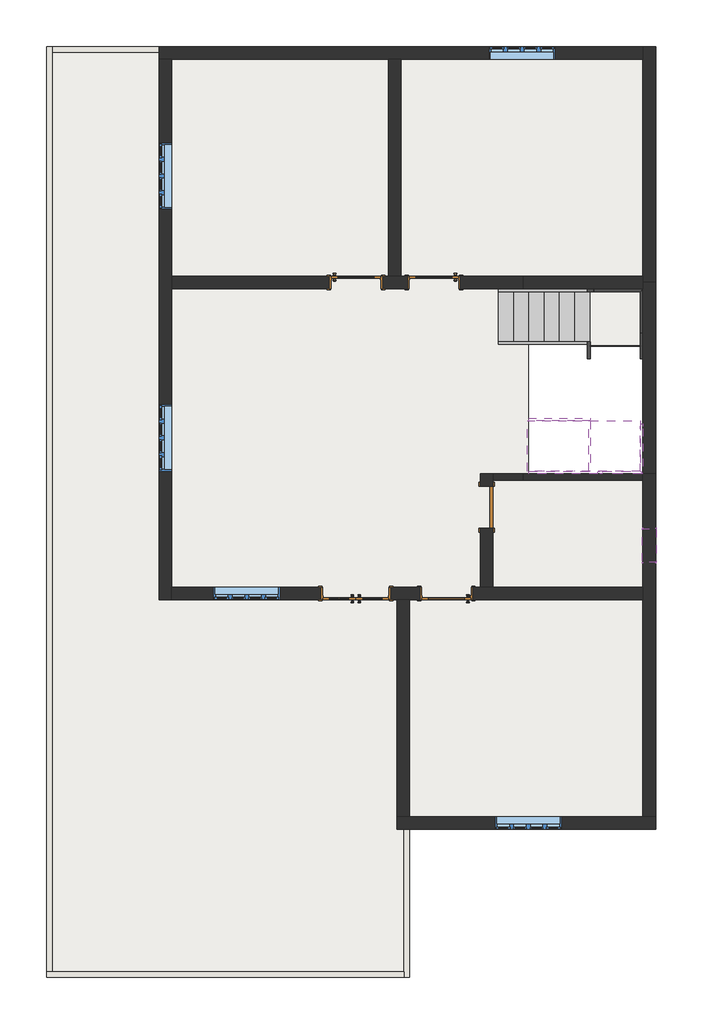
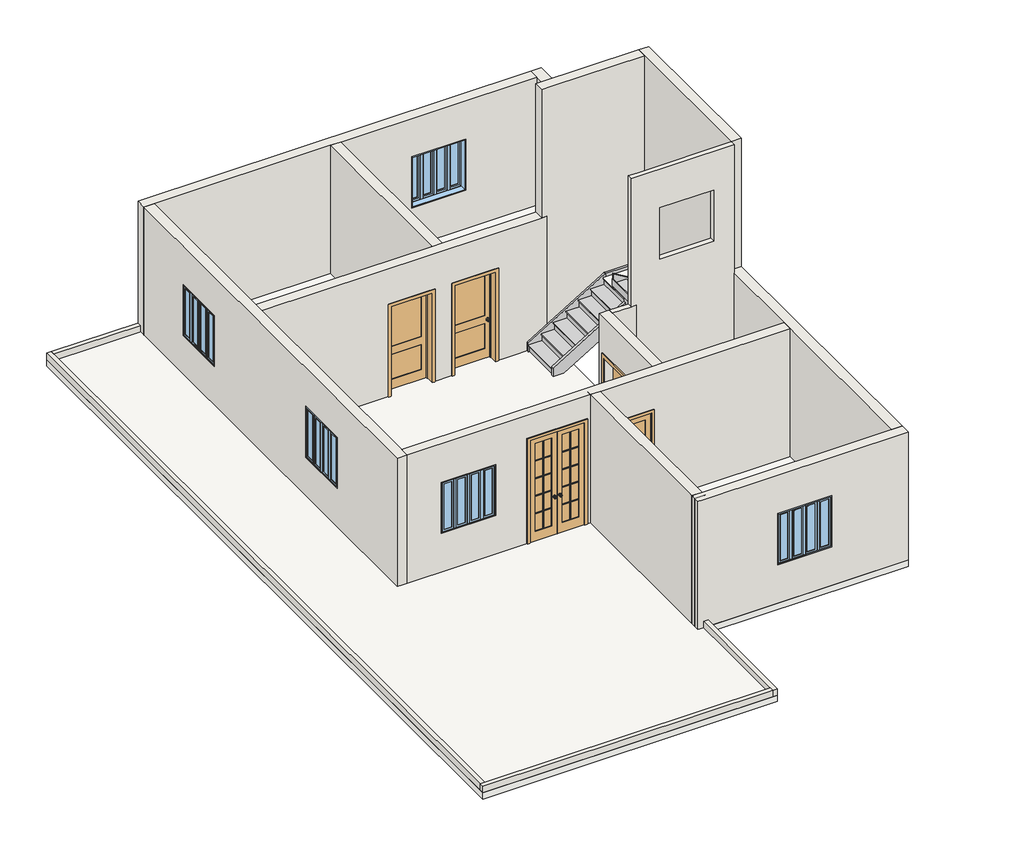
# One storey, incomplete: 18 walls, 10 members, 6 windows, 5 doors, 3 slabs, 3 stair flights, 2 columns.
"""IFC4 building model written with IfcOpenShell, lengths in millimetres."""

from ifc_helpers import new_model, si_unit, frame, origin, place, context, project, spatial, polyline, outline, extrude, faceted_brep, transform, mapped, element, save
from components import door_interior_double_full_glass_wood_4_x_8_door_7870f6d1, door_interior_single_2_panel_wood_3_x_7_door_08fe406f, door_interior_single_2_panel_wood_3_x_7_door_700963f9, door_e31f6e4d, non_monolithic_landing_e7e36702, non_monolithic_landing_8c0399ef, stair_flight_6437b1f2, stair_flight_4bd381d9, stair_flight_f110103f, window_casement_multi_sash_horizontal_4_x_4_8de01852, window_6da96920

model = new_model("IFC4")

# Units and contexts
model_context = context("Model", 3, world=origin())
ifc_project = project(units=[si_unit("LENGTHUNIT", "METRE", prefix="MILLI")], contexts=[model_context])

# Site, building, storey
site = spatial("IfcSite", under=ifc_project)
building = spatial("IfcBuilding", under=site)
storey = spatial("IfcBuildingStorey", under=building, Elevation=3048.0)

# Columns
placement = place(None, origin())
element("IfcColumn", 1, ObjectType="Rectangular Column : 9\" X 9\" COLUMN", at=placement, inside=storey, context=model_context, shape_type="SweptSolid", body=[
    extrude(outline(polyline([(-4334.4608498, -5108.7884134), (-4105.8608498, -5108.7884134), (-4105.8608498, -5222.3884134), (-4334.4608498, -5222.3884134), (-4334.4608498, -5108.7884134)])), frame((0.0, 0.0, 3048.0), z_axis=(0.0, 0.0, 1.0), x_axis=(1.0, 0.0, 0.0)), (0.0, 0.0, 1.0), 3048.0),
])
element("IfcColumn", 2, ObjectType="Rectangular Column : 9\" X 9\" COLUMN", at=placement, inside=storey, context=model_context, shape_type="SweptSolid", body=[
    extrude(outline(polyline([(-4105.8608498, -916.3884134), (-4105.8608498, -1144.9884134), (-4334.4608498, -1144.9884134), (-4334.4608498, -916.3884134), (-4105.8608498, -916.3884134)])), frame((0.0, 0.0, 3048.0), z_axis=(0.0, 0.0, 1.0), x_axis=(1.0, 0.0, 0.0)), (0.0, 0.0, 1.0), 3048.0),
])

# Doors
door_interior_double_full_glass_wood_4_x_8_door_shape = door_interior_double_full_glass_wood_4_x_8_door_7870f6d1(model_context)
element("IfcDoor", 3, ObjectType="Door-Interior-Double-Full Glass-Wood : 4' X 8' DOOR", at=placement, inside=storey, context=model_context, shape_type="MappedRepresentation", body=[
    mapped(door_interior_double_full_glass_wood_4_x_8_door_shape, transform((-5084.4608498, -1033.8634134, 3048.0), x_axis=(-1.0, 0.0, 0.0), y_axis=(0.0, -1.0, 0.0), z_axis=(0.0, 0.0, 1.0))),
])
door_interior_single_2_panel_wood_3_x_7_door_shape = door_interior_single_2_panel_wood_3_x_7_door_08fe406f(model_context)
element("IfcDoor", 4, ObjectType="Door-Interior-Single-2_Panel-Wood : 3' x 7' door", at=placement, inside=storey, context=model_context, shape_type="MappedRepresentation", body=[
    mapped(door_interior_single_2_panel_wood_3_x_7_door_shape, transform((-3430.6608498, -1033.8634134, 3048.0), x_axis=(-1.0, 0.0, 0.0), y_axis=(0.0, -1.0, 0.0), z_axis=(0.0, 0.0, 1.0))),
])
element("IfcDoor", 5, ObjectType="Door-Interior-Single-2_Panel-Wood : 3' x 7' door", at=placement, inside=storey, context=model_context, shape_type="MappedRepresentation", body=[
    mapped(door_interior_single_2_panel_wood_3_x_7_door_shape, transform((-5081.6608498, 4648.6865866, 3048.0), x_axis=(1.0, 0.0, 0.0), y_axis=(0.0, 1.0, 0.0), z_axis=(0.0, 0.0, 1.0))),
])
door_interior_single_2_panel_wood_3_x_7_door_2_shape = door_interior_single_2_panel_wood_3_x_7_door_700963f9(model_context)
element("IfcDoor", 6, ObjectType="Door-Interior-Single-2_Panel-Wood : 3' x 7' door", at=placement, inside=storey, context=model_context, shape_type="MappedRepresentation", body=[
    mapped(door_interior_single_2_panel_wood_3_x_7_door_2_shape, transform((-3657.8608498, 4648.6865866, 3048.0), x_axis=(-1.0, 0.0, 0.0), y_axis=(0.0, -1.0, 0.0), z_axis=(0.0, 0.0, 1.0))),
])
door_shape = door_e31f6e4d(model_context)
element("IfcDoor", 7, ObjectType="Single-Flush : 2'6\" x 7'", at=placement, inside=storey, context=model_context, shape_type="MappedRepresentation", body=[
    mapped(door_shape, transform((-2696.1608498, 542.7115866, 3048.0), x_axis=(0.0, 1.0, 0.0), y_axis=(-1.0, 0.0, 0.0), z_axis=(0.0, 0.0, 1.0))),
])

# Members
element("IfcMember", 8, ObjectType="Stringer - 2\" Width", at=placement, inside=storey, context=model_context, shape_type="SweptSolid", body=[
    extrude(outline(polyline([(3260.114512, -2479.5608498), (3048.0, -2479.5608498), (3048.0, -2241.475338), (4004.7333333, -662.865338), (4309.5333333, -748.0197945), (3260.114512, -2479.5608498)])), frame((0.0, 4479.7115866, 0.0), z_axis=(0.0, 1.0, 0.0), x_axis=(0.0, 0.0, 1.0)), (0.0, 0.0, 1.0), 50.8),
])
element("IfcMember", 9, ObjectType="Stringer - 2\" Width", at=placement, inside=storey, context=model_context, shape_type="SweptSolid", body=[
    extrude(outline(polyline([(3260.114512, -2479.5608498), (3048.0, -2479.5608498), (3048.0, -2241.475338), (3888.9178717, -853.9608498), (4245.3266332, -853.9608498), (3260.114512, -2479.5608498)])), frame((0.0, 3514.5115866, 0.0), z_axis=(0.0, 1.0, 0.0), x_axis=(0.0, 0.0, 1.0)), (0.0, 0.0, 1.0), 50.8),
])
element("IfcMember", 10, ObjectType="Stringer - 2\" Width", at=placement, inside=storey, context=model_context, shape_type="SweptSolid", body=[
    extrude(outline(polyline([(3738.7705314, 4309.5333333), (3653.6160748, 4004.7333333), (1977.2160748, 5020.7333333), (2062.3705314, 5325.5333333), (3738.7705314, 4309.5333333)])), frame((111.2391502, 0.0, 0.0), z_axis=(1.0, 0.0, 0.0), x_axis=(0.0, 1.0, 0.0)), (0.0, 0.0, 1.0), 50.8),
])
element("IfcMember", 11, ObjectType="Stringer - 2\" Width", at=placement, inside=storey, context=model_context, shape_type="Brep", body=[
    faceted_brep([(-803.1608498, 3565.3115866, 4414.6599665), (-853.9608498, 3565.3115866, 4414.6599665), (-853.9608498, 2168.3115866, 5261.3266332), (-803.1608498, 2168.3115866, 5261.3266332), (-803.1608498, 3565.3115866, 4058.251205), (-803.1608498, 2168.3115866, 5105.0390838), (-803.1608498, 2168.3115866, 4904.9178717), (-853.9608498, 3565.3115866, 4058.251205), (-853.9608498, 2168.3115866, 4904.9178717)], [[[0, 1, 2, 3]], [[4, 0, 3, 5, 6]], [[7, 4, 6, 8]], [[1, 7, 8, 2]], [[1, 0, 4, 7]], [[2, 8, 6, 5, 3]]]),
])
element("IfcMember", 12, ObjectType="Stringer - 2\" Width", at=placement, inside=storey, context=model_context, shape_type="Brep", body=[
    faceted_brep([(111.2391502, 3738.7705314, 4309.5333333), (162.0391502, 3738.7705314, 4309.5333333), (162.0391502, 4530.5115866, 4309.5333333), (111.2391502, 4479.7115866, 4309.5333333), (111.2391502, 3653.6160748, 4004.7333333), (111.2391502, 4479.7115866, 4004.7333333), (162.0391502, 3653.6160748, 4004.7333333), (162.0391502, 4530.5115866, 4004.7333333)], [[[0, 1, 2, 3]], [[4, 0, 3, 5]], [[6, 4, 5, 7]], [[1, 6, 7, 2]], [[1, 0, 4, 6]], [[2, 7, 5, 3]]]),
])
element("IfcMember", 13, ObjectType="Stringer - 2\" Width", at=placement, inside=storey, context=model_context, shape_type="Brep", body=[
    faceted_brep([(111.2391502, 4479.7115866, 4309.5333333), (162.0391502, 4530.5115866, 4309.5333333), (-748.0197945, 4530.5115866, 4309.5333333), (-748.0197945, 4479.7115866, 4309.5333333), (111.2391502, 4479.7115866, 4004.7333333), (-662.865338, 4479.7115866, 4004.7333333), (162.0391502, 4530.5115866, 4004.7333333), (-662.865338, 4530.5115866, 4004.7333333)], [[[0, 1, 2, 3]], [[4, 0, 3, 5]], [[6, 4, 5, 7]], [[1, 6, 7, 2]], [[1, 0, 4, 6]], [[2, 7, 5, 3]]]),
])
element("IfcMember", 14, ObjectType="Stringer - 2\" Width", at=placement, inside=storey, context=model_context, shape_type="SweptSolid", body=[
    extrude(outline(polyline([(5020.7333333, -664.0563615), (5325.5333333, -578.901905), (6138.7811786, -1920.7608498), (5782.3724171, -1920.7608498), (5020.7333333, -664.0563615)])), frame((0.0, 1152.3115866, 0.0), z_axis=(0.0, 1.0, 0.0), x_axis=(0.0, 0.0, 1.0)), (0.0, 0.0, 1.0), 50.8),
])
element("IfcMember", 15, ObjectType="Stringer - 2\" Width", at=placement, inside=storey, context=model_context, shape_type="Brep", body=[
    faceted_brep([(-1920.7608498, 2168.3115866, 6138.7811786), (-1920.7608498, 2168.3115866, 5782.3724171), (-1920.7608498, 2117.5115866, 5782.3724171), (-1920.7608498, 2117.5115866, 6138.7811786), (-803.1608498, 2117.5115866, 5461.4478453), (-803.1608498, 2168.3115866, 5461.4478453), (-803.1608498, 2117.5115866, 5105.0390838), (-803.1608498, 2168.3115866, 5105.0390838), (-803.1608498, 2168.3115866, 5261.3266332)], [[[0, 1, 2, 3]], [[4, 5, 0, 3]], [[6, 4, 3, 2]], [[7, 6, 2, 1]], [[5, 8, 7, 1, 0]], [[5, 4, 6, 7, 8]]]),
])
element("IfcMember", 16, ObjectType="Stringer - 2\" Width", at=placement, inside=storey, context=model_context, shape_type="Brep", body=[
    faceted_brep([(-578.901905, 1203.1115866, 5325.5333333), (-578.901905, 1152.3115866, 5325.5333333), (162.0391502, 1152.3115866, 5325.5333333), (111.2391502, 1203.1115866, 5325.5333333), (-664.0563615, 1203.1115866, 5020.7333333), (111.2391502, 1203.1115866, 5020.7333333), (-664.0563615, 1152.3115866, 5020.7333333), (162.0391502, 1152.3115866, 5020.7333333)], [[[0, 1, 2, 3]], [[4, 0, 3, 5]], [[6, 4, 5, 7]], [[1, 6, 7, 2]], [[1, 0, 4, 6]], [[2, 7, 5, 3]]]),
])
element("IfcMember", 17, ObjectType="Stringer - 2\" Width", at=placement, inside=storey, context=model_context, shape_type="Brep", body=[
    faceted_brep([(111.2391502, 1203.1115866, 5325.5333333), (162.0391502, 1152.3115866, 5325.5333333), (162.0391502, 2062.3705314, 5325.5333333), (111.2391502, 2062.3705314, 5325.5333333), (111.2391502, 1203.1115866, 5020.7333333), (111.2391502, 1977.2160748, 5020.7333333), (162.0391502, 1152.3115866, 5020.7333333), (162.0391502, 1977.2160748, 5020.7333333)], [[[0, 1, 2, 3]], [[4, 0, 3, 5]], [[6, 4, 5, 7]], [[1, 6, 7, 2]], [[1, 0, 4, 6]], [[2, 7, 5, 3]]]),
])

# Slabs
element("IfcSlab", 18, ObjectType="6\" FLOOR", at=placement, inside=storey, context=model_context, shape_type="SweptSolid", body=[
    extrude(outline(polyline([(-10733.1608498, 8952.9115866), (392.0391502, 8952.9115866), (392.0391502, -5337.3884134), (-4105.8608498, -5337.3884134), (-4105.8608498, -8043.1884134), (-10733.1608498, -8043.1884134), (-10733.1608498, 8952.9115866)]), holes=[polyline([(162.0391502, 1152.3115866), (162.0391502, 4530.5115866), (-1920.7608498, 4530.5115866), (-1920.7608498, 1152.3115866), (162.0391502, 1152.3115866)])]), frame((0.0, 0.0, 2895.6), z_axis=(0.0, 0.0, 1.0), x_axis=(1.0, 0.0, 0.0)), (0.0, 0.0, 1.0), 152.4),
])
non_monolithic_landing_shape = non_monolithic_landing_e7e36702(model_context)
element("IfcSlab", 19, ObjectType="Non-Monolithic Landing", at=placement, inside=storey, context=model_context, shape_type="MappedRepresentation", body=[
    mapped(non_monolithic_landing_shape, transform((0.0, 0.0, 0.0), x_axis=(1.0, 0.0, 0.0), y_axis=(0.0, 1.0, 0.0), z_axis=(0.0, 0.0, 1.0))),
])
non_monolithic_landing_2_shape = non_monolithic_landing_8c0399ef(model_context)
element("IfcSlab", 20, ObjectType="Non-Monolithic Landing", at=placement, inside=storey, context=model_context, shape_type="MappedRepresentation", body=[
    mapped(non_monolithic_landing_2_shape, transform((0.0, 0.0, 0.0), x_axis=(1.0, 0.0, 0.0), y_axis=(0.0, 1.0, 0.0), z_axis=(0.0, 0.0, 1.0))),
])

# Stair flights
stair_flight_shape = stair_flight_6437b1f2(model_context)
element("IfcStairFlight", 21, ObjectType="2\" Tread 1\" Nosing 1/4\" Riser", at=placement, inside=storey, context=model_context, shape_type="MappedRepresentation", body=[
    mapped(stair_flight_shape, transform((0.0, 0.0, 0.0), x_axis=(1.0, 0.0, 0.0), y_axis=(0.0, 1.0, 0.0), z_axis=(0.0, 0.0, 1.0))),
])
stair_flight_2_shape = stair_flight_4bd381d9(model_context)
element("IfcStairFlight", 22, ObjectType="2\" Tread 1\" Nosing 1/4\" Riser", at=placement, inside=storey, context=model_context, shape_type="MappedRepresentation", body=[
    mapped(stair_flight_2_shape, transform((0.0, 0.0, 0.0), x_axis=(1.0, 0.0, 0.0), y_axis=(0.0, 1.0, 0.0), z_axis=(0.0, 0.0, 1.0))),
])
stair_flight_3_shape = stair_flight_f110103f(model_context)
element("IfcStairFlight", 23, ObjectType="2\" Tread 1\" Nosing 1/4\" Riser", at=placement, inside=storey, context=model_context, shape_type="MappedRepresentation", body=[
    mapped(stair_flight_3_shape, transform((0.0, 0.0, 0.0), x_axis=(1.0, 0.0, 0.0), y_axis=(0.0, 1.0, 0.0), z_axis=(0.0, 0.0, 1.0))),
])

# Walls
element("IfcWall", 24, ObjectType="4\" wall", at=placement, inside=storey, context=model_context, shape_type="Brep", body=[
    faceted_brep([(-4207.4608498, -5338.0884134, 3048.0), (-4207.4608498, -7941.5884134, 3048.0), (-4207.4608498, -8043.1884134, 3048.0), (-4207.4608498, -8043.1884134, 3200.4), (-4207.4608498, -7941.5884134, 3200.4), (-4207.4608498, -5338.0884134, 3200.4), (-4105.8608498, -5338.0884134, 3048.0), (-4105.8608498, -5338.0884134, 3200.4), (-4105.8608498, -8043.1884134, 3200.4), (-4105.8608498, -8043.1884134, 3048.0)], [[[0, 1, 2, 3, 4, 5]], [[6, 7, 8, 9]], [[2, 1, 0, 6, 9]], [[5, 4, 3, 8, 7]], [[0, 5, 7, 6]], [[3, 2, 9, 8]]]),
])
element("IfcWall", 25, ObjectType="4\" wall", at=placement, inside=storey, context=model_context, shape_type="Brep", body=[
    faceted_brep([(-4207.4608498, -7941.5884134, 3048.0), (-10633.6608498, -7941.5884134, 3048.0), (-10735.2608498, -7941.5884134, 3048.0), (-10735.2608498, -7941.5884134, 3200.4), (-10633.6608498, -7941.5884134, 3200.4), (-4207.4608498, -7941.5884134, 3200.4), (-4207.4608498, -8043.1884134, 3048.0), (-4207.4608498, -8043.1884134, 3200.4), (-10735.2608498, -8043.1884134, 3200.4), (-10735.2608498, -8043.1884134, 3048.0)], [[[0, 1, 2, 3, 4, 5]], [[6, 7, 8, 9]], [[2, 1, 0, 6, 9]], [[5, 4, 3, 8, 7]], [[0, 5, 7, 6]], [[3, 2, 9, 8]]]),
])
element("IfcWall", 26, ObjectType="4\" wall", at=placement, inside=storey, context=model_context, shape_type="Brep", body=[
    faceted_brep([(-10633.6608498, -7941.5884134, 3048.0), (-10633.6608498, 8851.3115866, 3048.0), (-10633.6608498, 8952.9115866, 3048.0), (-10633.6608498, 8952.9115866, 3200.4), (-10633.6608498, 8851.3115866, 3200.4), (-10633.6608498, -7941.5884134, 3200.4), (-10735.2608498, -7941.5884134, 3048.0), (-10735.2608498, -7941.5884134, 3200.4), (-10735.2608498, 8952.9115866, 3200.4), (-10735.2608498, 8952.9115866, 3048.0)], [[[0, 1, 2, 3, 4, 5]], [[6, 7, 8, 9]], [[2, 1, 0, 6, 9]], [[5, 4, 3, 8, 7]], [[0, 5, 7, 6]], [[3, 2, 9, 8]]]),
])
element("IfcWall", 27, ObjectType="4\" wall", at=placement, inside=storey, context=model_context, shape_type="SweptSolid", body=[
    extrude(outline(polyline([(-8677.1608498, 8851.3115866), (-10633.6608498, 8851.3115866), (-10633.6608498, 8952.9115866), (-8677.1608498, 8952.9115866), (-8677.1608498, 8851.3115866)])), frame((0.0, 0.0, 3048.0), z_axis=(0.0, 0.0, 1.0), x_axis=(1.0, 0.0, 0.0)), (0.0, 0.0, 1.0), 152.4),
])
element("IfcWall", 28, ObjectType="4.5\" wall", at=placement, inside=storey, context=model_context, shape_type="Brep", body=[
    faceted_brep([(-2581.1608498, 1038.0115866, 3048.0), (-2035.7608498, 1038.0115866, 3048.0), (-2035.7608498, 1038.0115866, 6096.0), (-2150.7608498, 1038.0115866, 6096.0), (-2581.1608498, 1038.0115866, 6096.0), (-2581.1608498, 1152.3115866, 3048.0), (-2581.1608498, 1152.3115866, 6096.0), (-2150.7608498, 1152.3115866, 6096.0), (-2035.7608498, 1152.3115866, 6096.0), (-2035.7608498, 1152.3115866, 3048.0)], [[[0, 1, 2, 3, 4]], [[5, 6, 7, 8, 9]], [[1, 0, 5, 9]], [[2, 1, 9, 8]], [[4, 3, 2, 8, 7, 6]], [[0, 4, 6, 5]]]),
])
element("IfcWall", 29, ObjectType="4.5\" wall", at=placement, inside=storey, context=model_context, shape_type="Brep", body=[
    faceted_brep([(-2035.7608498, 1038.0115866, 3048.0), (162.0391502, 1038.0115866, 3048.0), (162.0391502, 1038.0115866, 9144.0), (-2150.7608498, 1038.0115866, 9144.0), (-2150.7608498, 1038.0115866, 6096.0), (-2035.7608498, 1038.0115866, 6096.0), (-1514.3608498, 1038.0115866, 8229.6), (-295.1608498, 1038.0115866, 8229.6), (-295.1608498, 1038.0115866, 7010.4), (-1514.3608498, 1038.0115866, 7010.4), (-2035.7608498, 1152.3115866, 3048.0), (-2035.7608498, 1152.3115866, 6096.0), (-2150.7608498, 1152.3115866, 6096.0), (-2150.7608498, 1152.3115866, 9144.0), (-1920.7608498, 1152.3115866, 9144.0), (162.0391502, 1152.3115866, 9144.0), (162.0391502, 1152.3115866, 3048.0), (-1514.3608498, 1152.3115866, 8229.6), (-1514.3608498, 1152.3115866, 7010.4), (-295.1608498, 1152.3115866, 7010.4), (-295.1608498, 1152.3115866, 8229.6)], [[[0, 1, 2, 3, 4, 5], [6, 7, 8, 9]], [[10, 11, 12, 13, 14, 15, 16], [17, 18, 19, 20]], [[1, 0, 10, 16]], [[3, 2, 15, 14, 13]], [[2, 1, 16, 15]], [[0, 5, 11, 10]], [[4, 12, 11, 5]], [[4, 3, 13, 12]], [[18, 17, 6, 9]], [[19, 18, 9, 8]], [[20, 19, 8, 7]], [[17, 20, 7, 6]]]),
])
element("IfcWall", 30, ObjectType="9\" wall", at=placement, inside=storey, context=model_context, shape_type="Brep", body=[
    faceted_brep([(-4335.1608498, -5338.0884134, 3048.0), (-4207.4608498, -5338.0884134, 3048.0), (-4105.8608498, -5338.0884134, 3048.0), (392.0391502, -5338.0884134, 3048.0), (392.0391502, -5338.0884134, 6096.0), (-4220.1608498, -5338.0884134, 6096.0), (-4335.1608498, -5338.0884134, 6096.0), (-2542.3608498, -5338.0884134, 5181.6), (-1323.1608498, -5338.0884134, 5181.6), (-1323.1608498, -5338.0884134, 3962.4), (-2542.3608498, -5338.0884134, 3962.4), (-4335.1608498, -5108.0884134, 3048.0), (-4335.1608498, -5108.0884134, 6096.0), (-4105.1608498, -5108.0884134, 6096.0), (162.0391502, -5108.0884134, 6096.0), (392.0391502, -5108.0884134, 6096.0), (392.0391502, -5108.0884134, 3048.0), (162.0391502, -5108.0884134, 3048.0), (-4105.1608498, -5108.0884134, 3048.0), (-2542.3608498, -5108.0884134, 5181.6), (-2542.3608498, -5108.0884134, 3962.4), (-1323.1608498, -5108.0884134, 3962.4), (-1323.1608498, -5108.0884134, 5181.6)], [[[0, 1, 2, 3, 4, 5, 6], [7, 8, 9, 10]], [[11, 12, 13, 14, 15, 16, 17, 18], [19, 20, 21, 22]], [[3, 2, 1, 0, 11, 18, 17, 16]], [[6, 5, 4, 15, 14, 13, 12]], [[4, 3, 16, 15]], [[0, 6, 12, 11]], [[20, 19, 7, 10]], [[21, 20, 10, 9]], [[22, 21, 9, 8]], [[19, 22, 8, 7]]]),
])
element("IfcWall", 31, ObjectType="9\" wall", at=placement, inside=storey, context=model_context, shape_type="Brep", body=[
    faceted_brep([(392.0391502, -5108.0884134, 3048.0), (392.0391502, 1155.1115866, 3048.0), (392.0391502, 1155.1115866, 6096.0), (392.0391502, -5108.0884134, 6096.0), (392.0391502, 151.1115866, 5181.6), (392.0391502, 151.1115866, 4572.0), (392.0391502, -458.4884134, 4572.0), (392.0391502, -458.4884134, 5181.6), (162.0391502, -5108.0884134, 3048.0), (162.0391502, -5108.0884134, 6096.0), (162.0391502, -1145.6884134, 6096.0), (162.0391502, -915.6884134, 6096.0), (162.0391502, 1155.1115866, 6096.0), (162.0391502, 1155.1115866, 3048.0), (162.0391502, 1152.3115866, 3048.0), (162.0391502, 1038.0115866, 3048.0), (162.0391502, -915.6884134, 3048.0), (162.0391502, -1145.6884134, 3048.0), (162.0391502, 151.1115866, 5181.6), (162.0391502, -458.4884134, 5181.6), (162.0391502, -458.4884134, 4572.0), (162.0391502, 151.1115866, 4572.0), (290.4391502, 1155.1115866, 6096.0)], [[[0, 1, 2, 3], [4, 5, 6, 7]], [[8, 9, 10, 11, 12, 13, 14, 15, 16, 17], [18, 19, 20, 21]], [[1, 0, 8, 17, 16, 15, 14, 13]], [[2, 1, 13, 12, 22]], [[3, 2, 22, 12, 11, 10, 9]], [[0, 3, 9, 8]], [[5, 4, 18, 21]], [[6, 5, 21, 20]], [[7, 6, 20, 19]], [[4, 7, 19, 18]]]),
])
element("IfcWall", 32, ObjectType="9\" wall", at=placement, inside=storey, context=model_context, shape_type="Brep", body=[
    faceted_brep([(162.0391502, 8952.9115866, 3048.0), (-8677.1608498, 8952.9115866, 3048.0), (-8677.1608498, 8952.9115866, 3200.4), (-8677.1608498, 8952.9115866, 6096.0), (162.0391502, 8952.9115866, 6096.0), (-1436.7608498, 8952.9115866, 5181.6), (-2655.9608498, 8952.9115866, 5181.6), (-2655.9608498, 8952.9115866, 3962.4), (-1436.7608498, 8952.9115866, 3962.4), (162.0391502, 8722.9115866, 3048.0), (162.0391502, 8722.9115866, 6096.0), (-4254.7608498, 8722.9115866, 6096.0), (-4484.7608498, 8722.9115866, 6096.0), (-8447.1608498, 8722.9115866, 6096.0), (-8677.1608498, 8722.9115866, 6096.0), (-8677.1608498, 8722.9115866, 3048.0), (-8447.1608498, 8722.9115866, 3048.0), (-4484.7608498, 8722.9115866, 3048.0), (-4254.7608498, 8722.9115866, 3048.0), (-1436.7608498, 8722.9115866, 5181.6), (-1436.7608498, 8722.9115866, 3962.4), (-2655.9608498, 8722.9115866, 3962.4), (-2655.9608498, 8722.9115866, 5181.6), (-8677.1608498, 8851.3115866, 3048.0)], [[[0, 1, 2, 3, 4], [5, 6, 7, 8]], [[9, 10, 11, 12, 13, 14, 15, 16, 17, 18], [19, 20, 21, 22]], [[1, 0, 9, 18, 17, 16, 15, 23]], [[4, 3, 14, 13, 12, 11, 10]], [[0, 4, 10, 9]], [[20, 19, 5, 8]], [[21, 20, 8, 7]], [[22, 21, 7, 6]], [[19, 22, 6, 5]], [[1, 23, 15, 14, 3, 2]]]),
])
element("IfcWall", 33, ObjectType="9\" wall", at=placement, inside=storey, context=model_context, shape_type="Brep", body=[
    faceted_brep([(-8677.1608498, 8722.9115866, 6096.0), (-8677.1608498, 8722.9115866, 3048.0), (-8677.1608498, -1145.6884134, 3048.0), (-8677.1608498, -1145.6884134, 6096.0), (-8677.1608498, 7198.9115866, 5181.6), (-8677.1608498, 5979.7115866, 5181.6), (-8677.1608498, 5979.7115866, 3962.4), (-8677.1608498, 7198.9115866, 3962.4), (-8677.1608498, 2417.0115866, 5181.6), (-8677.1608498, 1197.8115866, 5181.6), (-8677.1608498, 1197.8115866, 3962.4), (-8677.1608498, 2417.0115866, 3962.4), (-8447.1608498, 8722.9115866, 3048.0), (-8447.1608498, 8722.9115866, 6096.0), (-8447.1608498, 4760.5115866, 6096.0), (-8447.1608498, 4530.5115866, 6096.0), (-8447.1608498, -915.6884134, 6096.0), (-8447.1608498, -1145.6884134, 6096.0), (-8447.1608498, -1145.6884134, 3048.0), (-8447.1608498, -915.6884134, 3048.0), (-8447.1608498, 4530.5115866, 3048.0), (-8447.1608498, 4760.5115866, 3048.0), (-8447.1608498, 7198.9115866, 5181.6), (-8447.1608498, 7198.9115866, 3962.4), (-8447.1608498, 5979.7115866, 3962.4), (-8447.1608498, 5979.7115866, 5181.6), (-8447.1608498, 2417.0115866, 5181.6), (-8447.1608498, 2417.0115866, 3962.4), (-8447.1608498, 1197.8115866, 3962.4), (-8447.1608498, 1197.8115866, 5181.6)], [[[0, 1, 2, 3], [4, 5, 6, 7], [8, 9, 10, 11]], [[12, 13, 14, 15, 16, 17, 18, 19, 20, 21], [22, 23, 24, 25], [26, 27, 28, 29]], [[2, 1, 12, 21, 20, 19, 18]], [[0, 3, 17, 16, 15, 14, 13]], [[3, 2, 18, 17]], [[23, 22, 4, 7]], [[24, 23, 7, 6]], [[25, 24, 6, 5]], [[22, 25, 5, 4]], [[27, 26, 8, 11]], [[28, 27, 11, 10]], [[29, 28, 10, 9]], [[26, 29, 9, 8]], [[0, 13, 12, 1]]]),
])
element("IfcWall", 34, ObjectType="9\" wall", at=placement, inside=storey, context=model_context, shape_type="Brep", body=[
    faceted_brep([(162.0391502, 4760.5115866, 9144.0), (162.0391502, 4760.5115866, 6096.0), (162.0391502, 4760.5115866, 3048.0), (-2035.7608498, 4760.5115866, 3048.0), (-2035.7608498, 4760.5115866, 6096.0), (-2150.7608498, 4760.5115866, 6096.0), (-2150.7608498, 4760.5115866, 9144.0), (162.0391502, 4530.5115866, 3048.0), (162.0391502, 4530.5115866, 9144.0), (-1920.7608498, 4530.5115866, 9144.0), (-2150.7608498, 4530.5115866, 9144.0), (-2150.7608498, 4530.5115866, 6096.0), (-2035.7608498, 4530.5115866, 6096.0), (-2035.7608498, 4530.5115866, 3048.0), (162.0391502, 4645.5115866, 3048.0)], [[[0, 1, 2, 3, 4, 5, 6]], [[7, 8, 9, 10, 11, 12, 13]], [[3, 2, 14, 7, 13]], [[0, 6, 10, 9, 8]], [[4, 3, 13, 12]], [[11, 5, 4, 12]], [[6, 5, 11, 10]], [[0, 8, 7, 14, 2, 1]]]),
])
element("IfcWall", 35, ObjectType="9\" wall", at=placement, inside=storey, context=model_context, shape_type="SweptSolid", body=[
    extrude(outline(polyline([(-4484.7608498, 4760.5115866), (-4484.7608498, 8722.9115866), (-4254.7608498, 8722.9115866), (-4254.7608498, 4760.5115866), (-4484.7608498, 4760.5115866)])), frame((0.0, 0.0, 3048.0), z_axis=(0.0, 0.0, 1.0), x_axis=(1.0, 0.0, 0.0)), (0.0, 0.0, 1.0), 3048.0),
])
element("IfcWall", 36, ObjectType="9\" wall", at=placement, inside=storey, context=model_context, shape_type="Brep", body=[
    faceted_brep([(162.0391502, -1145.6884134, 6096.0), (-4105.1608498, -1145.6884134, 6096.0), (-4335.1608498, -1145.6884134, 6096.0), (-8447.1608498, -1145.6884134, 6096.0), (-8447.1608498, -1145.6884134, 3048.0), (-5719.4608498, -1145.6884134, 3048.0), (-5719.4608498, -1145.6884134, 5511.8), (-4449.4608498, -1145.6884134, 5511.8), (-4449.4608498, -1145.6884134, 3048.0), (-4335.1608498, -1145.6884134, 3048.0), (-4105.1608498, -1145.6884134, 3048.0), (-3913.2608498, -1145.6884134, 3048.0), (-3913.2608498, -1145.6884134, 5207.0), (-2948.0608498, -1145.6884134, 5207.0), (-2948.0608498, -1145.6884134, 3048.0), (162.0391502, -1145.6884134, 3048.0), (-7685.1608498, -1145.6884134, 5181.6), (-6465.9608498, -1145.6884134, 5181.6), (-6465.9608498, -1145.6884134, 3962.4), (-7685.1608498, -1145.6884134, 3962.4), (-8447.1608498, -915.6884134, 6096.0), (-2811.1608498, -915.6884134, 6096.0), (-2581.1608498, -915.6884134, 6096.0), (162.0391502, -915.6884134, 6096.0), (162.0391502, -915.6884134, 3048.0), (-2581.1608498, -915.6884134, 3048.0), (-2811.1608498, -915.6884134, 3048.0), (-2948.0608498, -915.6884134, 3048.0), (-2948.0608498, -915.6884134, 5207.0), (-3913.2608498, -915.6884134, 5207.0), (-3913.2608498, -915.6884134, 3048.0), (-4449.4608498, -915.6884134, 3048.0), (-4449.4608498, -915.6884134, 5511.8), (-5719.4608498, -915.6884134, 5511.8), (-5719.4608498, -915.6884134, 3048.0), (-8447.1608498, -915.6884134, 3048.0), (-7685.1608498, -915.6884134, 5181.6), (-7685.1608498, -915.6884134, 3962.4), (-6465.9608498, -915.6884134, 3962.4), (-6465.9608498, -915.6884134, 5181.6)], [[[0, 1, 2, 3, 4, 5, 6, 7, 8, 9, 10, 11, 12, 13, 14, 15], [16, 17, 18, 19]], [[20, 21, 22, 23, 24, 25, 26, 27, 28, 29, 30, 31, 32, 33, 34, 35], [36, 37, 38, 39]], [[24, 15, 14, 27, 26, 25]], [[4, 35, 34, 5]], [[30, 11, 10, 9, 8, 31]], [[3, 2, 1, 0, 23, 22, 21, 20]], [[0, 15, 24, 23]], [[4, 3, 20, 35]], [[29, 12, 11, 30]], [[12, 29, 28, 13]], [[13, 28, 27, 14]], [[37, 36, 16, 19]], [[38, 37, 19, 18]], [[39, 38, 18, 17]], [[36, 39, 17, 16]], [[33, 6, 5, 34]], [[6, 33, 32, 7]], [[7, 32, 31, 8]]]),
])
element("IfcWall", 37, ObjectType="9\" wall", at=placement, inside=storey, context=model_context, shape_type="SweptSolid", body=[
    extrude(outline(polyline([(-4105.1608498, -1145.6884134), (-4105.1608498, -5108.0884134), (-4335.1608498, -5108.0884134), (-4335.1608498, -1145.6884134), (-4105.1608498, -1145.6884134)])), frame((0.0, 0.0, 3048.0), z_axis=(0.0, 0.0, 1.0), x_axis=(1.0, 0.0, 0.0)), (0.0, 0.0, 1.0), 3048.0),
])
element("IfcWall", 38, ObjectType="9\" wall", at=placement, inside=storey, context=model_context, shape_type="Brep", body=[
    faceted_brep([(-2811.1608498, 1152.3115866, 3048.0), (-2811.1608498, 923.7115866, 3048.0), (-2811.1608498, 923.7115866, 5181.6), (-2811.1608498, 161.7115866, 5181.6), (-2811.1608498, 161.7115866, 3048.0), (-2811.1608498, -915.6884134, 3048.0), (-2811.1608498, -915.6884134, 6096.0), (-2811.1608498, 1152.3115866, 6096.0), (-2581.1608498, 923.7115866, 5181.6), (-2581.1608498, 923.7115866, 3048.0), (-2581.1608498, 1038.0115866, 3048.0), (-2581.1608498, 1152.3115866, 3048.0), (-2581.1608498, 1152.3115866, 6096.0), (-2581.1608498, 1038.0115866, 6096.0), (-2581.1608498, -915.6884134, 6096.0), (-2581.1608498, -915.6884134, 3048.0), (-2581.1608498, 161.7115866, 3048.0), (-2581.1608498, 161.7115866, 5181.6)], [[[0, 1, 2, 3, 4, 5, 6, 7]], [[8, 9, 10, 11, 12, 13, 14, 15, 16, 17]], [[16, 15, 5, 4]], [[11, 10, 9, 1, 0]], [[7, 6, 14, 13, 12]], [[6, 5, 15, 14]], [[0, 7, 12, 11]], [[2, 1, 9, 8]], [[3, 2, 8, 17]], [[4, 3, 17, 16]]]),
])
element("IfcWall", 39, ObjectType="9\" wall", at=placement, inside=storey, context=model_context, shape_type="Brep", body=[
    faceted_brep([(392.0391502, 4645.5115866, 3048.0), (392.0391502, 8952.9115866, 3048.0), (392.0391502, 8952.9115866, 6096.0), (392.0391502, 4760.5115866, 6096.0), (392.0391502, 4645.5115866, 6096.0), (162.0391502, 4645.5115866, 3048.0), (162.0391502, 4645.5115866, 6096.0), (162.0391502, 4760.5115866, 6096.0), (162.0391502, 8722.9115866, 6096.0), (162.0391502, 8952.9115866, 6096.0), (162.0391502, 8952.9115866, 3048.0), (162.0391502, 8722.9115866, 3048.0), (162.0391502, 4760.5115866, 3048.0)], [[[0, 1, 2, 3, 4]], [[5, 6, 7, 8, 9, 10, 11, 12]], [[1, 0, 5, 12, 11, 10]], [[4, 3, 2, 9, 8, 7, 6]], [[0, 4, 6, 5]], [[2, 1, 10, 9]]]),
])
element("IfcWall", 40, ObjectType="9\" wall", at=placement, inside=storey, context=model_context, shape_type="Brep", body=[
    faceted_brep([(392.0391502, 1155.1115866, 9144.0), (392.0391502, 1155.1115866, 6248.4), (392.0391502, 1155.1115866, 6096.0), (392.0391502, 1155.1115866, 3048.0), (392.0391502, 4645.5115866, 3048.0), (392.0391502, 4645.5115866, 6096.0), (392.0391502, 4760.5115866, 6096.0), (392.0391502, 4760.5115866, 6248.4), (392.0391502, 4760.5115866, 9144.0), (162.0391502, 1155.1115866, 3048.0), (162.0391502, 1155.1115866, 6096.0), (162.0391502, 1155.1115866, 9144.0), (162.0391502, 4530.5115866, 9144.0), (162.0391502, 4760.5115866, 9144.0), (162.0391502, 4760.5115866, 6096.0), (162.0391502, 4645.5115866, 6096.0), (162.0391502, 4645.5115866, 3048.0), (162.0391502, 4530.5115866, 3048.0), (290.4391502, 4760.5115866, 6096.0)], [[[0, 1, 2, 3, 4, 5, 6, 7, 8]], [[9, 10, 11, 12, 13, 14, 15, 16, 17]], [[4, 3, 9, 17, 16]], [[0, 8, 13, 12, 11]], [[0, 11, 10, 9, 3, 2, 1]], [[5, 4, 16, 15]], [[14, 18, 6, 5, 15]], [[6, 18, 14, 13, 8, 7]]]),
])
element("IfcWall", 41, ObjectType="9\" wall", at=placement, inside=storey, context=model_context, shape_type="Brep", body=[
    faceted_brep([(-8447.1608498, 4760.5115866, 6096.0), (-4484.7608498, 4760.5115866, 6096.0), (-4254.7608498, 4760.5115866, 6096.0), (-2150.7608498, 4760.5115866, 6096.0), (-2035.7608498, 4760.5115866, 6096.0), (-2035.7608498, 4760.5115866, 3048.0), (-3175.2608498, 4760.5115866, 3048.0), (-3175.2608498, 4760.5115866, 5207.0), (-4140.4608498, 4760.5115866, 5207.0), (-4140.4608498, 4760.5115866, 3048.0), (-4254.7608498, 4760.5115866, 3048.0), (-4484.7608498, 4760.5115866, 3048.0), (-4599.0608498, 4760.5115866, 3048.0), (-4599.0608498, 4760.5115866, 5207.0), (-5564.2608498, 4760.5115866, 5207.0), (-5564.2608498, 4760.5115866, 3048.0), (-8447.1608498, 4760.5115866, 3048.0), (-2035.7608498, 4530.5115866, 6096.0), (-2150.7608498, 4530.5115866, 6096.0), (-8447.1608498, 4530.5115866, 6096.0), (-8447.1608498, 4530.5115866, 3048.0), (-5564.2608498, 4530.5115866, 3048.0), (-5564.2608498, 4530.5115866, 5207.0), (-4599.0608498, 4530.5115866, 5207.0), (-4599.0608498, 4530.5115866, 3048.0), (-4140.4608498, 4530.5115866, 3048.0), (-4140.4608498, 4530.5115866, 5207.0), (-3175.2608498, 4530.5115866, 5207.0), (-3175.2608498, 4530.5115866, 3048.0), (-2035.7608498, 4530.5115866, 3048.0)], [[[0, 1, 2, 3, 4, 5, 6, 7, 8, 9, 10, 11, 12, 13, 14, 15, 16]], [[17, 18, 19, 20, 21, 22, 23, 24, 25, 26, 27, 28, 29]], [[20, 16, 15, 21]], [[24, 12, 11, 10, 9, 25]], [[5, 29, 28, 6]], [[4, 3, 2, 1, 0, 19, 18, 17]], [[5, 4, 17, 29]], [[0, 16, 20, 19]], [[23, 13, 12, 24]], [[13, 23, 22, 14]], [[14, 22, 21, 15]], [[8, 26, 25, 9]], [[26, 8, 7, 27]], [[27, 7, 6, 28]]]),
])

# Windows
window_casement_multi_sash_horizontal_4_x_4_shape = window_casement_multi_sash_horizontal_4_x_4_8de01852(model_context)
element("IfcWindow", 42, ObjectType="Window-Casement-Multi-Sash-Horizontal : 4' x 4'", at=placement, inside=storey, context=model_context, shape_type="MappedRepresentation", body=[
    mapped(window_casement_multi_sash_horizontal_4_x_4_shape, transform((-8562.1608498, 6589.3115866, 3048.0), x_axis=(0.0, 1.0, 0.0), y_axis=(-1.0, 0.0, 0.0), z_axis=(0.0, 0.0, 1.0))),
])
element("IfcWindow", 43, ObjectType="Window-Casement-Multi-Sash-Horizontal : 4' x 4'", at=placement, inside=storey, context=model_context, shape_type="MappedRepresentation", body=[
    mapped(window_casement_multi_sash_horizontal_4_x_4_shape, transform((-2046.3608498, 8837.9115866, 3048.0), x_axis=(1.0, 0.0, 0.0), y_axis=(0.0, 1.0, 0.0), z_axis=(0.0, 0.0, 1.0))),
])
element("IfcWindow", 44, ObjectType="Window-Casement-Multi-Sash-Horizontal : 4' x 4'", at=placement, inside=storey, context=model_context, shape_type="MappedRepresentation", body=[
    mapped(window_casement_multi_sash_horizontal_4_x_4_shape, transform((-8562.1608498, 1807.4115866, 3048.0), x_axis=(0.0, 1.0, 0.0), y_axis=(-1.0, 0.0, 0.0), z_axis=(0.0, 0.0, 1.0))),
])
element("IfcWindow", 45, ObjectType="Window-Casement-Multi-Sash-Horizontal : 4' x 4'", at=placement, inside=storey, context=model_context, shape_type="MappedRepresentation", body=[
    mapped(window_casement_multi_sash_horizontal_4_x_4_shape, transform((-7075.5608498, -1030.6884134, 3048.0), x_axis=(-1.0, 0.0, 0.0), y_axis=(0.0, -1.0, 0.0), z_axis=(0.0, 0.0, 1.0))),
])
element("IfcWindow", 46, ObjectType="Window-Casement-Multi-Sash-Horizontal : 4' x 4'", at=placement, inside=storey, context=model_context, shape_type="MappedRepresentation", body=[
    mapped(window_casement_multi_sash_horizontal_4_x_4_shape, transform((-1932.7608498, -5223.0884134, 3048.0), x_axis=(-1.0, 0.0, 0.0), y_axis=(0.0, -1.0, 0.0), z_axis=(0.0, 0.0, 1.0))),
])
window_shape = window_6da96920(model_context)
element("IfcWindow", 47, ObjectType="Window-Louvers : 24\" x 24\"", at=placement, inside=storey, context=model_context, shape_type="MappedRepresentation", body=[
    mapped(window_shape, transform((283.3891502, -153.6884134, 3657.6), x_axis=(0.0, -1.0, 0.0), y_axis=(1.0, 0.0, 0.0), z_axis=(0.0, 0.0, 1.0))),
])

save(model, "model.ifc")

# Revit data of these elements
# Type "Rectangular Column : 9\" X 9\" COLUMN"
#   Assembly Code = "B1010200"
#   Depth = 0' - 9"
#   Offset Base = 0' - 0"
#   Offset Top = 0' - 0"
#   Width = 0' - 9"
#   Material = none
# Type "Door-Interior-Double-Full Glass-Wood : 4' X 8' DOOR"
#   Type Mark = "12"
#   Assembly Code = "C1020300"
#   Analytic Construction = "French door, wood frame with single glass"
#   Top Rail = 0' - 4 11/16"
#   Thickness = 0' - 1 3/8"
#   Thermal Resistance (R) = 1.0696 (h·ft²·°F)/BTU
#   Swing Angle [instance default] = 90.00°
#   Stiles = 0' - 4 3/4"
#   Rough Width = 4' - 2"
#   Rough Height = 8' - 1"
#   Panel Width = 2' - 0"
#   Height = 8' - 0"
#   Width = 4' - 0"
#   Heat Transfer Coefficient (U) = 0.9350 BTU/(h·ft²·°F)
#   Bottom Rail = 0' - 9 1/8"
#   Show Grill [instance default] = yes
#   Trim Material = Cherry
#   Panel Material = Cherry
#   Frame Material = Cherry
#   Door Handle Material = Aluminum
#   Visual Light Transmittance = 0
#   Solar Heat Gain Coefficient = 0
#   Wall Closure = (empty or 0)
#   Function = (empty or 0)
# Type "Door-Interior-Single-2_Panel-Wood : 3' x 7' door"
#   Type Mark = "9"
#   Assembly Code = "C1020300"
#   Analytic Construction = "Wooden"
#   Top Rail = 0' - 4 11/16"
#   Thickness = 0' - 1 3/8"
#   Thermal Resistance (R) = 2.5876 (h·ft²·°F)/BTU
#   Swing Angle [instance default] = 90.00°
#   Stiles = 0' - 4 3/4"
#   Rough Width = 3' - 2"
#   Rough Height = 7' - 1"
#   Lock Rail = 0' - 7 1/2"
#   Height = 7' - 0"
#   Width = 3' - 0"
#   Heat Transfer Coefficient (U) = 0.3865 BTU/(h·ft²·°F)
#   Bottom Rail = 0' - 9 1/8"
#   Trim Material = Cherry
#   Panel Material = Cherry
#   Frame Material = Cherry
#   Door Handle Material = Aluminum
#   Visual Light Transmittance = 0
#   Solar Heat Gain Coefficient = 0
#   Wall Closure = (empty or 0)
#   Function = (empty or 0)
# Type "Single-Flush : 2'6\" x 7'"
#   Type Mark = "10"
#   Construction Type Id = "MDOOR"
#   Assembly Code = "C1020"
#   Analytic Construction = "Metal"
#   Thickness = 0' - 2"
#   Heat Transfer Coefficient (U) = 0.651978 BTU/(h·ft²·°F)
#   Height = 7' - 0"
#   Trim Projection Ext = 0' - 1"
#   Trim Projection Int = 0' - 1"
#   Trim Width = 0' - 3"
#   Width = 2' - 6"
#   Define Thermal Properties by = 1
#   Door Material = Door - Panel
#   Frame Material = Door - Frame
#   Visual Light Transmittance = 0
#   Solar Heat Gain Coefficient = 0
#   Function = (empty or 0)
#   Wall Closure = (empty or 0)
# Type "6\" FLOOR"
#   Assembly Code = "B1010"
#   Function = 0
#   Layers, outside or top first: 0' - 6" no material (function 1)
# Type "4\" wall"
#   Assembly Code = "B2010"
#   Layers, outside or top first: 0' - 4" no material (function 1)
# Type "4.5\" wall"
#   Assembly Code = "B2010"
#   Layers, outside or top first: 0' - 4 1/2" no material (function 1)
# Type "9\" wall"
#   Assembly Code = "B2010"
#   Layers, outside or top first: 0' - 9 7/128" no material (function 1)
# Type "Window-Casement-Multi-Sash-Horizontal : 4' x 4'"
#   Type Mark = "W1"
#   Fire Rating = "0.5h"
#   Assembly Code = "B2020100"
#   Analytic Construction = "Double glazing - domestic"
#   Window Inset [instance default] = 0' - 0 5/8"
#   Wall Thickness [instance default] = 0' - 6"
#   Visual Light Transmittance = 0.81
#   Thermal Resistance (R) = 1.8146 (h·ft²·°F)/BTU
#   Solar Heat Gain Coefficient = 0.76
#   Rough Width = 4' - 0 1/2"
#   Rough Height = 4' - 0 1/2"
#   Open Window Width = 1' - 0"
#   Heat Transfer Coefficient (U) = 0.5511 BTU/(h·ft²·°F)
#   Height = 4' - 0"
#   Frame Gap 3 [instance default] = 0' - 1 83/128"
#   Frame Gap 2 [instance default] = 0' - 0 5/8"
#   Frame Gap 1 = 0' - 1 51/128"
#   Default Sill Height = 3' - 0"
#   Width = 4' - 0"
#   Frame Material = Metal - Aluminum
#   Glass Panel Material = Glass
#   Wall Closure = (empty or 0)
# Type "Window-Louvers : 24\" x 24\""
#   Type Mark = "V"
#   Construction Type Id = "GSP4R"
#   Assembly Code = "B20"
#   Analytic Construction = "1/8 in Pilkington single glazing"
#   Visual Light Transmittance = 0.9
#   Thermal Resistance (R) = 1.53941 (h·ft²·°F)/BTU
#   Solar Heat Gain Coefficient = 0.78
#   Max Height = 1' - 11.74264"
#   Height = 2' - 0"
#   Heat Transfer Coefficient (U) = 0.6496 BTU/(h·ft²·°F)
#   Blade Width [instance default] = 1' - 10 1/2"
#   Blade Vertical Thickness = 0' - 0.35355"
#   Blade Thickness = 0' - 0 1/4"
#   Blade Spacing = 0' - 1 1/2"
#   Blade Height = 0' - 1.85355"
#   Blade Depth = 0' - 3"
#   Blade Angle = 45.00°
#   Default Sill Height = 3' - 0"
#   Trim Projection_Exterior = 0' - 0 1/2"
#   Trim Projection_Interior = 0' - 0 1/2"
#   Trim Width_Exterior = 0' - 1 1/2"
#   Trim Width_Interior = 0' - 1 1/2"
#   Width = 2' - 0"
#   Max Blade Count = 12
#   Define Thermal Properties by = 1
#   Blade Count = 12
#   Frame Material = Birch
#   Louver Material = Birch
#   Trim Exterior Material = Birch
#   Trim Interior Material = Birch
#   Wall Closure = (empty or 0)
# Element 1 (IfcColumn, "Rectangular Column : 9\" X 9\" COLUMN")
#   Phase Created = New Construction
#   Materials on its faces: "Default Wall"
# Element 2 (IfcColumn, "Rectangular Column : 9\" X 9\" COLUMN")
#   Phase Created = New Construction
# Element 3 (IfcDoor, "Door-Interior-Double-Full Glass-Wood : 4' X 8' DOOR")
#   Swing Angle = 90.00°
#   Show Grill = yes
#   Phase Created = New Construction
#   Materials on its faces: "Cherry", "Aluminum", "Glass"
# Elements 4, 5, 6 (IfcDoor, "Door-Interior-Single-2_Panel-Wood : 3' x 7' door")
#   Swing Angle = 90.00°
#   Phase Created = New Construction
#   Materials on its faces: "Cherry", "Aluminum"
# Element 7 (IfcDoor, "Single-Flush : 2'6\" x 7'")
#   Phase Created = New Construction
#   Materials on its faces: "Door - Frame", "Door - Panel"
# Elements 8, 9, 10, 11, 12, 13, 14, 15, 16, 17 (IfcMember, "Stringer - 2\" Width")
#   Phase Created = New Construction
# Element 18 (IfcSlab, "6\" FLOOR")
#   built-in parameter 1001955 = 3.14159 (stored number, unit not read)
#   Height Offset From Level = 0' - 0"
#   Phase Created = New Construction
#   Materials on its faces: "Default Floor", "white colour"
# Elements 19, 20 (IfcSlab, "Non-Monolithic Landing")
#   Phase Created = New Construction
# Elements 21, 22, 23 (IfcStairFlight, "2\" Tread 1\" Nosing 1/4\" Riser")
#   Phase Created = New Construction
# Elements 24, 27 (IfcWall, "4\" wall")
#   Top Offset = 0' - 0"
#   Base Offset = 0' - 0"
#   Unconnected Height = 0' - 6"
#   wall height = 0' - 6"
#   Phase Created = New Construction
#   Materials on its faces: "Default Wall", "white colour"
# Elements 25, 26 (IfcWall, "4\" wall")
#   Top Offset = 0' - 0"
#   Base Offset = 0' - 0"
#   Unconnected Height = 0' - 6"
#   wall height = 0' - 6"
#   Phase Created = New Construction
#   Materials on its faces: "white colour", "Default Wall"
# Element 28 (IfcWall, "4.5\" wall")
#   Top Offset = 0' - 0"
#   Base Offset = 0' - 0"
#   Unconnected Height = 10' - 0"
#   wall height = 10' - 0"
#   Phase Created = New Construction
#   Materials on its faces: "Default Wall"
# Element 29 (IfcWall, "4.5\" wall")
#   Top Offset = 0' - 0"
#   Base Offset = 0' - 0"
#   wall height = 20' - 0"
#   Phase Created = New Construction
#   Materials on its faces: "Default Wall", "white colour", "Main wall"
# Element 30 (IfcWall, "9\" wall")
#   Top Offset = 0' - 0"
#   Base Offset = 0' - 0"
#   Unconnected Height = 10' - 0"
#   wall height = 10' - 0"
#   Phase Created = New Construction
#   Materials on its faces: "Default Wall", "Natural stone", "white colour", "Main wall"
# Elements 31, 39 (IfcWall, "9\" wall")
#   Top Offset = 0' - 0"
#   Base Offset = 0' - 0"
#   Unconnected Height = 10' - 0"
#   wall height = 10' - 0"
#   Phase Created = New Construction
#   Materials on its faces: "Default Wall", "white colour"
# Element 32 (IfcWall, "9\" wall")
#   Top Offset = 0' - 0"
#   Base Offset = 0' - 0"
#   Unconnected Height = 10' - 0"
#   wall height = 10' - 0"
#   Phase Created = New Construction
#   Materials on its faces: "Default Wall", "white colour", "Main wall"
# Elements 33, 36, 37 (IfcWall, "9\" wall")
#   Top Offset = 0' - 0"
#   Base Offset = 0' - 0"
#   Unconnected Height = 10' - 0"
#   wall height = 10' - 0"
#   Phase Created = New Construction
#   Materials on its faces: "Default Wall", "Main wall"
# Element 34 (IfcWall, "9\" wall")
#   Top Offset = 0' - 0"
#   Base Offset = 0' - 0"
#   wall height = 20' - 0"
#   Phase Created = New Construction
#   Materials on its faces: "Default Wall", "Main wall"
# Elements 35, 38, 41 (IfcWall, "9\" wall")
#   Top Offset = 0' - 0"
#   Base Offset = 0' - 0"
#   Unconnected Height = 10' - 0"
#   wall height = 10' - 0"
#   Phase Created = New Construction
#   Materials on its faces: "Default Wall"
# Element 40 (IfcWall, "9\" wall")
#   Top Offset = 0' - 0"
#   Base Offset = 0' - 0"
#   Unconnected Height = 20' - 0"
#   wall height = 20' - 0"
#   Phase Created = New Construction
#   Materials on its faces: "Default Wall", "Main wall"
# Element 42 (IfcWindow, "Window-Casement-Multi-Sash-Horizontal : 4' x 4'")
#   Mark = "7"
#   Window Inset = 0' - 0 5/8"
#   Frame Gap 3 = 0' - 1 83/128"
#   Frame Gap 2 = 0' - 0 5/8"
#   Phase Created = New Construction
#   Materials on its faces: "Metal - Aluminum", "Glass"
# Element 43 (IfcWindow, "Window-Casement-Multi-Sash-Horizontal : 4' x 4'")
#   Mark = "8"
#   Window Inset = 0' - 0 5/8"
#   Frame Gap 3 = 0' - 1 83/128"
#   Frame Gap 2 = 0' - 0 5/8"
#   Phase Created = New Construction
#   Materials on its faces: "Metal - Aluminum", "Glass"
# Element 44 (IfcWindow, "Window-Casement-Multi-Sash-Horizontal : 4' x 4'")
#   Mark = "9"
#   Window Inset = 0' - 0 5/8"
#   Frame Gap 3 = 0' - 1 83/128"
#   Frame Gap 2 = 0' - 0 5/8"
#   Phase Created = New Construction
#   Materials on its faces: "Metal - Aluminum", "Glass"
# Element 45 (IfcWindow, "Window-Casement-Multi-Sash-Horizontal : 4' x 4'")
#   Mark = "10"
#   Window Inset = 0' - 0 5/8"
#   Frame Gap 3 = 0' - 1 83/128"
#   Frame Gap 2 = 0' - 0 5/8"
#   Phase Created = New Construction
#   Materials on its faces: "Metal - Aluminum", "Glass"
# Element 46 (IfcWindow, "Window-Casement-Multi-Sash-Horizontal : 4' x 4'")
#   Mark = "11"
#   Window Inset = 0' - 0 5/8"
#   Frame Gap 3 = 0' - 1 83/128"
#   Frame Gap 2 = 0' - 0 5/8"
#   Phase Created = New Construction
#   Materials on its faces: "Metal - Aluminum", "Glass"
# Element 47 (IfcWindow, "Window-Louvers : 24\" x 24\"")
#   Mark = "12"
#   Blade Width = 1' - 10 1/2"
#   Phase Created = New Construction
#   Materials on its faces: "Birch"
# Materials
#   "Cherry": class "Wood", colour RGB 226 177 128, transparency 0, Description = "Prunus Serotina", Cost = 0
#   "Aluminum": class "Metal", colour RGB 247 247 247, transparency 0, Description = "Aluminum 6061", Cost = 0
#   "Door - Panel": class "Wood", colour RGB 210 159 95, transparency 0, Cost = 0
#   "Door - Frame": colour RGB 118 70 51, transparency 0, Cost = 0
#   "Metal - Aluminum": class "Metal", colour RGB 247 247 247, transparency 0
#   "Glass": class "Glass", colour RGB 0 128 192, transparency 0.75, Description = "Soda Lime Glass", Cost = 0
#   "Birch": class "Wood", colour RGB 224 178 126, transparency 0, Description = "Betula Alleghaniensis", Cost = 0
#   "Default Wall": colour RGB 128 128 128, transparency 0, Cost = 0
#   "Default Floor": colour RGB 128 128 128, transparency 0, Cost = 0
#   "white colour": class "Generic", colour RGB 120 120 120, transparency 0, Cost = 0
#   "Main wall": class "Generic", colour RGB 120 120 120, transparency 0, Cost = 0
#   "Natural stone": class "Generic", colour RGB 120 120 120, transparency 0, Cost = 0
